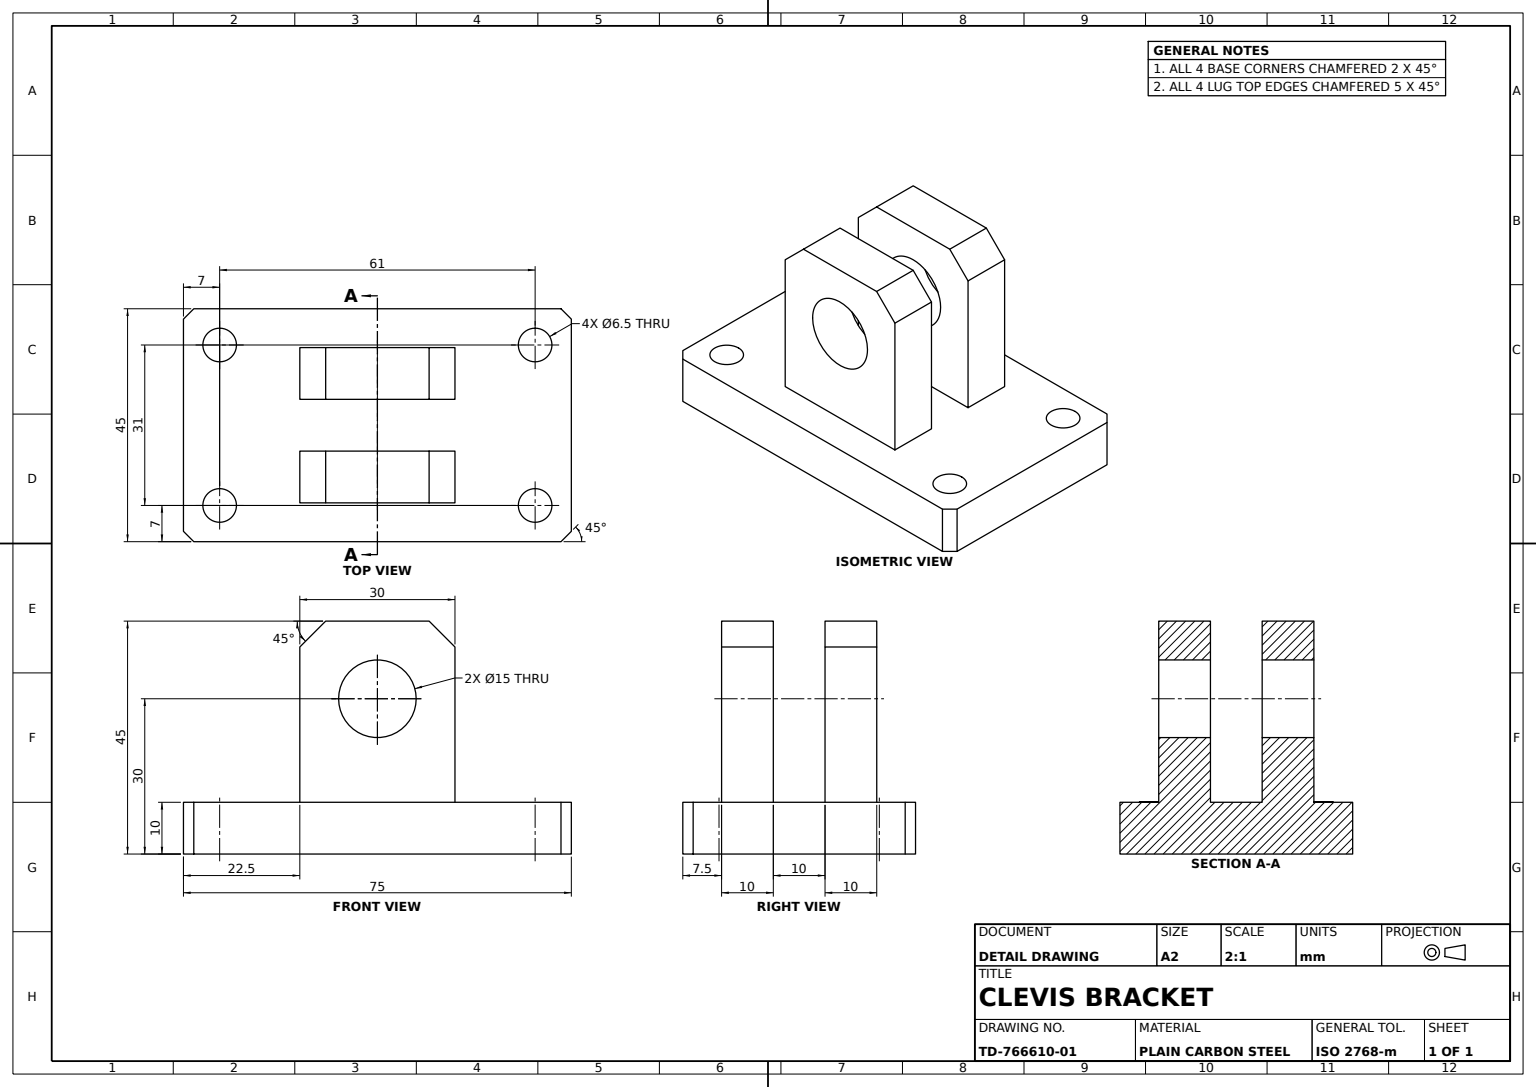
from build123d import *

# Parameters (mm, degrees)
BASE_PLATE_SKETCH_W        = 75
BASE_PLATE_SKETCH_H        = 45
BASE_PLATE_75X45X10_DEPTH  = 10
BASE_CORNER_CHAMFER_1_SIZE = 2
BASE_CORNER_CHAMFER_2_SIZE = 2
BASE_CORNER_CHAMFER_3_SIZE = 2
BASE_CORNER_CHAMFER_4_SIZE = 2
FORK_BODY_SKETCH_W         = 30
FORK_BODY_SKETCH_H         = 35
FORK_BODY_SKETCH_R         = 7.5
FORK_BODY_DEPTH            = 10
FORK_EXTENSION_SKETCH_W    = 30
FORK_EXTENSION_SKETCH_H    = 35
FORK_EXTENSION_SKETCH_R    = 7.5
FORK_EXTENSION_DEPTH       = 17.5
FORK_SLOT_SKETCH_W         = 30
FORK_SLOT_SKETCH_H         = 35
FORK_SLOT_SKETCH_R         = 7.5
FORK_SLOT_DEPTH            = 7.5
FORK_TOP_CHAMFER_1_SIZE    = 5
FORK_TOP_CHAMFER_2_SIZE    = 5
MOUNTING_HOLES_SKETCH_R    = 3.25
MOUNTING_HOLES_DEPTH       = 57.013391256


with BuildPart() as part:
    # Base Plate Sketch → Base Plate 75x45x10 (new body)
    with BuildSketch(Plane(origin=(0, 0, 0), x_dir=(1, 0, 0), z_dir=(0, 1, 0))):
        Rectangle(BASE_PLATE_SKETCH_W, BASE_PLATE_SKETCH_H)
    extrude(amount=BASE_PLATE_75X45X10_DEPTH)

    # Base Corner Chamfer 1
    base_corner_chamfer_1_edges = [part.edges().sort_by_distance(p)[0] for p in [
        (37.5, 5, 22.5),
    ]]
    chamfer(base_corner_chamfer_1_edges, length=BASE_CORNER_CHAMFER_1_SIZE)

    # Base Corner Chamfer 2
    base_corner_chamfer_2_edges = [part.edges().sort_by_distance(p)[0] for p in [
        (-37.5, 5, 22.5),
    ]]
    chamfer(base_corner_chamfer_2_edges, length=BASE_CORNER_CHAMFER_2_SIZE)

    # Base Corner Chamfer 3
    base_corner_chamfer_3_edges = [part.edges().sort_by_distance(p)[0] for p in [
        (-37.5, 5, -22.5),
    ]]
    chamfer(base_corner_chamfer_3_edges, length=BASE_CORNER_CHAMFER_3_SIZE)

    # Base Corner Chamfer 4
    base_corner_chamfer_4_edges = [part.edges().sort_by_distance(p)[0] for p in [
        (37.5, 5, -22.5),
    ]]
    chamfer(base_corner_chamfer_4_edges, length=BASE_CORNER_CHAMFER_4_SIZE)

    # Fork Body Sketch → Fork Body (add)
    with BuildSketch(Plane.XY.offset(5)):
        with Locations((0, 27.5)):
            Rectangle(FORK_BODY_SKETCH_W, FORK_BODY_SKETCH_H)
        with Locations((0, 30)):
            Circle(FORK_BODY_SKETCH_R, mode=Mode.SUBTRACT)
    extrude(amount=FORK_BODY_DEPTH)

    # Fork Extension Sketch → Fork Extension (add)
    with BuildSketch(Plane(origin=(0, 0, -22.5), x_dir=(-1, 0, 0), z_dir=(0, 0, -1))):
        with Locations((0, 27.5)):
            Rectangle(FORK_EXTENSION_SKETCH_W, FORK_EXTENSION_SKETCH_H)
        with Locations(Location((0, 30, 0), (0, 0, 180))):
            Circle(FORK_EXTENSION_SKETCH_R, mode=Mode.SUBTRACT)
    extrude(amount=-FORK_EXTENSION_DEPTH)

    # Fork Slot Sketch → Fork Slot (cut)
    with BuildSketch(Plane(origin=(0, 0, -22.5), x_dir=(-1, 0, 0), z_dir=(0, 0, -1))):
        with Locations((0, 27.5)):
            Rectangle(FORK_SLOT_SKETCH_W, FORK_SLOT_SKETCH_H)
        with Locations(Location((0, 30, 0), (0, 0, 180))):
            Circle(FORK_SLOT_SKETCH_R, mode=Mode.SUBTRACT)
    extrude(amount=-FORK_SLOT_DEPTH, mode=Mode.SUBTRACT)

    # Fork Top Chamfer 1
    fork_top_chamfer_1_edges = [part.edges().sort_by_distance(p)[0] for p in [
        (-15, 45, -10),
    ]]
    chamfer(fork_top_chamfer_1_edges, length=FORK_TOP_CHAMFER_1_SIZE)

    # Fork Top Chamfer 2
    fork_top_chamfer_2_edges = [part.edges().sort_by_distance(p)[0] for p in [
        (15, 45, 10),
        (-15, 45, 10),
        (15, 45, -10),
    ]]
    chamfer(fork_top_chamfer_2_edges, length=FORK_TOP_CHAMFER_2_SIZE)

    # Mounting Holes Sketch → Mounting Holes (cut, through all)
    with BuildSketch(Plane(origin=(0, 10, 0), x_dir=(1, 0, 0), z_dir=(0, 1, 0))):
        with Locations(Location((-30.5, 15.5, 0), (0, 0, 270))):
            Circle(MOUNTING_HOLES_SKETCH_R)
        with Locations(Location((-30.5, -15.5, 0), (0, 0, 270))):
            Circle(MOUNTING_HOLES_SKETCH_R)
        with Locations(Location((30.5, -15.5, 0), (0, 0, 90))):
            Circle(MOUNTING_HOLES_SKETCH_R)
        with Locations(Location((30.5, 15.5, 0), (0, 0, 90))):
            Circle(MOUNTING_HOLES_SKETCH_R)
    extrude(amount=-MOUNTING_HOLES_DEPTH, mode=Mode.SUBTRACT)


solid = part.part
